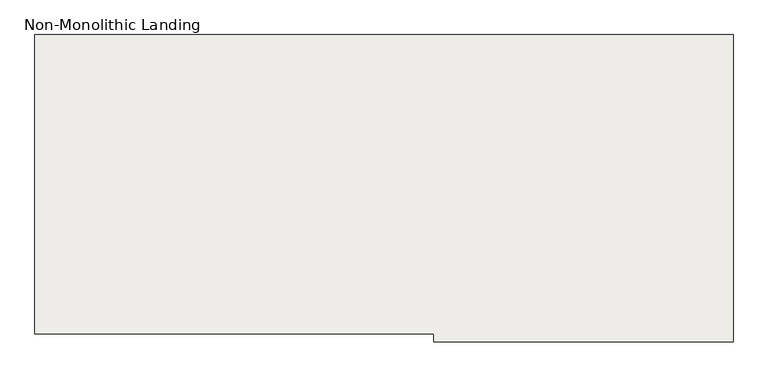
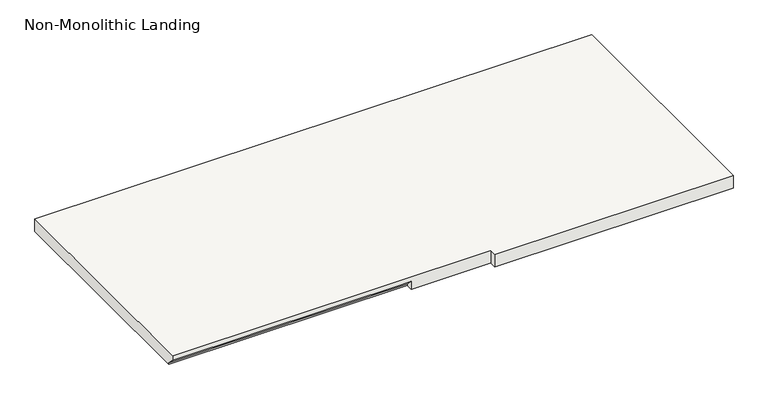
"""IFC4 building model written with IfcOpenShell, lengths in millimetres: slab geometry, Non-Monolithic Landing."""

from ifc_helpers import new_model, si_unit, origin, place, context, project, spatial, faceted_brep, source, transform, mapped, element, save


def non_monolithic_landing_abd20321(model_context):
    return source(origin(), model_context, "Body", "Brep", [
        faceted_brep([(-3617.4415084, 23194.7216096, 39608.9005799), (-3617.4415084, 23220.1216096, 39583.5005799), (-2703.0415084, 23220.1216096, 39583.5005799), (-2703.0415084, 23194.7216096, 39608.9005799), (-2398.2415084, 23194.7216096, 39627.9505799), (-2398.2415084, 23169.3216096, 39627.9505799), (-1483.8415084, 23169.3216096, 39627.9505799), (-1483.8415084, 23194.7216096, 39627.9505799), (-1483.8415084, 24109.1216096, 39627.9505799), (-3617.4415084, 24109.1216096, 39627.9505799), (-3617.4415084, 23194.7216096, 39627.9505799), (-2703.0415084, 23220.1216096, 39577.1505799), (-3617.4415084, 23220.1216096, 39577.1505799), (-3617.4415084, 24109.1216096, 39577.1505799), (-1483.8415084, 24109.1216096, 39577.1505799), (-1483.8415084, 23194.7216096, 39577.1505799), (-1483.8415084, 23169.3216096, 39577.1505799), (-2398.2415084, 23169.3216096, 39577.1505799), (-2398.2415084, 23194.7216096, 39577.1505799), (-2703.0415084, 23194.7216096, 39577.1505799)], [[[0, 1, 2, 3]], [[4, 5, 6, 7, 8, 9, 10]], [[11, 12, 13, 14, 15, 16, 17, 18, 19]], [[12, 11, 2, 1]], [[11, 19, 3, 2]], [[4, 10, 0, 3, 19, 18]], [[5, 4, 18, 17]], [[6, 5, 17, 16]], [[7, 6, 16, 15]], [[8, 7, 15, 14]], [[9, 8, 14, 13]], [[10, 9, 13, 12, 1, 0]]]),
    ])


if __name__ == "__main__":
    model = new_model("IFC4")
    model_context = context("Model", 3, world=origin())
    ifc_project = project(units=[si_unit("LENGTHUNIT", "METRE", prefix="MILLI")], contexts=[model_context])
    site = spatial("IfcSite", under=ifc_project)
    building = spatial("IfcBuilding", under=site)
    placement = place(None, origin())
    non_monolithic_landing_shape = non_monolithic_landing_abd20321(model_context)
    element("IfcSlab", 1, ObjectType="Non-Monolithic Landing", at=placement, inside=building, context=model_context, shape_type="MappedRepresentation", body=[
        mapped(non_monolithic_landing_shape, transform((0.0, 0.0, 0.0), x_axis=(1.0, 0.0, 0.0), y_axis=(0.0, 1.0, 0.0), z_axis=(0.0, 0.0, 1.0))),
    ])
    save(model, "model.ifc")
